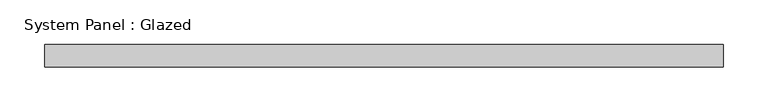
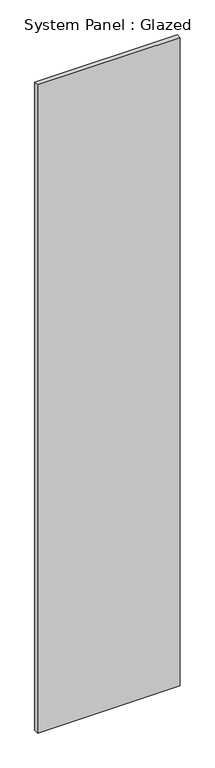
"""IFC4 building model written with IfcOpenShell, lengths in millimetres: plate geometry, System Panel : Glazed."""

from ifc_helpers import new_model, si_unit, origin, origin_with_axes, place, context, project, spatial, polyline, outline, extrude, source, transform, mapped, element, save


def system_panel_glazed_20dba380(model_context):
    return source(origin(), model_context, "Body", "SweptSolid", [
        extrude(outline(polyline([(381.0, 19.05), (-381.0, 19.05), (-381.0, 44.45), (381.0, 44.45), (381.0, 19.05)])), origin_with_axes(), (0.0, 0.0, 1.0), 3657.6),
    ])


if __name__ == "__main__":
    model = new_model("IFC4")
    model_context = context("Model", 3, world=origin())
    ifc_project = project(units=[si_unit("LENGTHUNIT", "METRE", prefix="MILLI")], contexts=[model_context])
    site = spatial("IfcSite", under=ifc_project)
    building = spatial("IfcBuilding", under=site)
    placement = place(None, origin())
    system_panel_glazed_shape = system_panel_glazed_20dba380(model_context)
    element("IfcPlate", 1, ObjectType="System Panel : Glazed", at=placement, inside=building, context=model_context, shape_type="MappedRepresentation", body=[
        mapped(system_panel_glazed_shape, transform((0.0, 0.0, 0.0), x_axis=(1.0, 0.0, 0.0), y_axis=(0.0, 1.0, 0.0), z_axis=(0.0, 0.0, 1.0))),
    ])
    save(model, "model.ifc")

# Revit data of these elements
# Type "System Panel : Glazed"
#   Construction Type Id = "GSP4R"
#   Analytic Construction = "1/8 in Pilkington single glazing"
#   Visual Light Transmittance = 0.9
#   Solar Heat Gain Coefficient = 0.86
#   Heat Transfer Coefficient (U) = 1.18115 BTU/(h·ft²·°F)
# Element 1 (IfcPlate, "System Panel : Glazed")
#   Materials on its faces: "Glass"
# Materials
#   "Glass": class "Glass", colour RGB 0 128 192, transparency 0.75, Description = "Soda Lime Glass", Cost = 0
